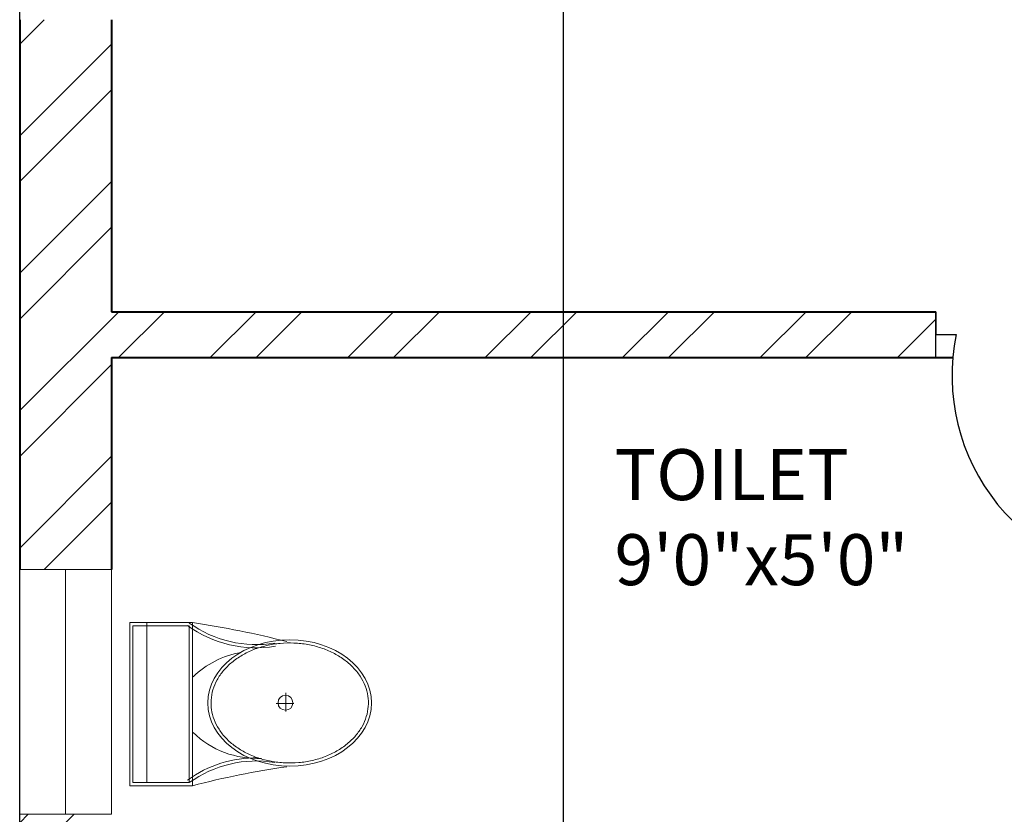
# Model space of a CAD drawing. Units: inches. Extents: x 1601 to 2297, y 1496 to 2631.
# Tile 6 of 57: x 1686 to 1783, y 1835 to 1913. Entities that reach past the tile are written whole.
import ezdxf

# ---------------------------------------------------------------- set-up
doc = ezdxf.new("R2010")
doc.units = ezdxf.units.IN
for name, color, linetype, lineweight in [('A-ANNO-DIMS', 2, 'Continuous', 18), ('A-AREA-IDEN', 7, 'Continuous', 18), ('A-DOOR', 21, 'Continuous', 25), ('A-FLOR-FIXT', 9, 'Continuous', 20), ('A-GLAZ', 161, 'Continuous', 20), ('A-WALL', 7, 'Continuous', 40), ('A-WALL-PATT', 215, 'Continuous', 13)]:
    doc.layers.add(name, color=color, linetype=linetype, lineweight=lineweight)
doc.styles.get("Standard").update_dxf_attribs({"font": 'arial.ttf'})
doc.dimstyles.get("Standard").update_dxf_attribs({"dimtxt": 0.18, "dimasz": 0.18, "dimexe": 0.18, "dimexo": 0.0625, "dimgap": 0.09, "dimtad": 0, "dimtih": 1, "dimtoh": 1, "dimdec": 4, "dimzin": 0, "dimdsep": 46, "dimtxsty": 'Standard', "dimcen": 0.09, "dimadec": 0, "dimazin": 0, "dimtfac": 1, "dimtdec": 4, "dimtofl": 0, "dimtmove": 0, "dimatfit": 3, "dimfxl": 1, "dimtolj": 1, "dimtzin": 0, "dimarcsym": 0})

# ---------------------------------------------------------------- blocks, each defined once
blk = doc.blocks.new('A$C31115884')
for p, q in [((257.5, 466.4), (257.5, 523.2)), ((283.1, 497.7), (223.4, 497.7)), ((0, 200), (0, 0)), ((520, 200), (0, 200)), ((10, 190), (10, 10)), ((510, 190), (10, 190)), ((510, 10), (510, 190)), ((520, 0), (520, 200)), ((510, 54.5), (0, 54.5)), ((10, 10), (510, 10)), ((0, 0), (520, 0))]:
    blk.add_line(p, q)
blk.add_circle((255.6, 496.4), 23.6)
for centre, radius, start, end in [((2777.7, -204.6), 2807, 165.4549, 171.7133), ((3237, 905), 2807, 188.2867, 194.5451), ((-294.5, 403.3), 364.7, 324.2091, 9.3499), ((-294.5, 403.3), 374.7, 324.2091, 9.3499), ((805.8, 403.3), 364.7, 170.6501, 215.7909), ((139.5, 406.2), 293.5, 315.8436, 2.6563), ((805.8, 403.3), 374.7, 179.2036, 215.7909), ((383.6, 406.2), 293.5, 190.2774, 224.1564)]:
    blk.add_arc(centre, radius, start, end)
blk.add_ellipse((256.2, 509.9), major_axis=(0, -260.7), ratio=0.772727)
blk.add_open_spline([(256.2, 259.2), (263.1, 259.2), (270, 259.7), (287.8, 262.3), (298.7, 265.1), (319.9, 273.1), (330.2, 278.4), (350.1, 291.1), (359.7, 298.7), (377.7, 315.9), (386.2, 325.5), (401.7, 346.6), (408.8, 358.1), (421.3, 382.5), (426.8, 395.5), (435.9, 422.4), (439.5, 436.4), (444.8, 465.1), (446.5, 479.7), (447.9, 509.2), (447.6, 524), (445, 553.3), (442.7, 567.8), (436.3, 596), (432.1, 609.7), (421.9, 636), (416, 648.6), (402.5, 672.1), (395, 683), (378.6, 703), (369.8, 712.1), (351.1, 728), (341.3, 734.8), (320.9, 746.2), (310.4, 750.7), (288.9, 757.3), (278, 759.4), (256, 761), (245, 760.6), (223.1, 757.2), (212.3, 754.3), (191.1, 746.1), (180.8, 740.7), (160.9, 727.8), (151.4, 720.1), (133.5, 702.7), (125.1, 693), (109.6, 671.7), (102.6, 660.2), (90.2, 635.7), (84.9, 622.7), (76, 595.6), (72.4, 581.6), (67.2, 552.9), (65.6, 538.2), (64.4, 508.8), (64.8, 494), (67.5, 464.7), (69.9, 450.2), (76.6, 422), (80.8, 408.3), (91.1, 382.2), (97.2, 369.7), (110.8, 346.3), (118.4, 335.4), (134.8, 315.6), (143.7, 306.7), (162.4, 290.9), (172.3, 284.2), (192.8, 273), (203.3, 268.6), (224.8, 262.2), (235.8, 260.2), (249.9, 259.3), (253, 259.2), (256.2, 259.2)], degree=3, knots=[0, 0, 0, 0, 0.110105, 0.110105, 0.285049, 0.285049, 0.459994, 0.459994, 0.634938, 0.634938, 0.809882, 0.809882, 0.984827, 0.984827, 1.159771, 1.159771, 1.334715, 1.334715, 1.50966, 1.50966, 1.684604, 1.684604, 1.859549, 1.859549, 2.034493, 2.034493, 2.209437, 2.209437, 2.384382, 2.384382, 2.559326, 2.559326, 2.73427, 2.73427, 2.909215, 2.909215, 3.084159, 3.084159, 3.259103, 3.259103, 3.434048, 3.434048, 3.608992, 3.608992, 3.783936, 3.783936, 3.958881, 3.958881, 4.133825, 4.133825, 4.30877, 4.30877, 4.483714, 4.483714, 4.658658, 4.658658, 4.833603, 4.833603, 5.008547, 5.008547, 5.183491, 5.183491, 5.358436, 5.358436, 5.53338, 5.53338, 5.708324, 5.708324, 5.883269, 5.883269, 6.058213, 6.058213, 6.233158, 6.233158, 6.283185, 6.283185, 6.283185, 6.283185])
blk = doc.blocks.new('WIN-24IN-JAMB9')
for p, q in [((4.5, 24), (0, 24)), ((0, 24), (9, 24)), ((0, 24), (0, 0)), ((4.5, 0), (4.5, 24)), ((9, 24), (9, 0)), ((0, 0), (9, 0)), ((9, 0), (4.5, 0))]:
    blk.add_line(p, q)
blk = doc.blocks.new('*D36')
at = {"layer": 'A-ANNO-DIMS', "color": 0, "lineweight": -2, "transparency": 16777216}
for p, q in [((1686.037, 1635.388), (1686.037, 2581.055)), ((1739.334, 1635.388), (1739.334, 2581.055)), ((1686.217, 2580.875), (1712.362, 2580.875)), ((1739.154, 2580.875), (1713.009, 2580.875))]:
    blk.add_line(p, q, dxfattribs=at)
at = {"layer": 'A-ANNO-DIMS', "color": 0, "transparency": 16777216}
for points in [[(1686.217, 2580.905), (1686.217, 2580.845), (1686.037, 2580.875)], [(1739.154, 2580.905), (1739.154, 2580.845), (1739.334, 2580.875)]]:
    blk.add_solid(points, dxfattribs=at)
at = {"layer": 'Defpoints', "color": 0, "transparency": 16777216}
for p in [(1739.334, 2580.875), (1686.037, 1635.325), (1739.334, 1635.325)]:
    blk.add_point(p, dxfattribs=at)
at = {"layer": 'A-ANNO-DIMS', "color": 0, "transparency": 16777216, "insert": (1712.685, 2580.875), "char_height": 0.18, "attachment_point": 5}
blk.add_mtext('\\A1;53.3', dxfattribs=at)

msp = doc.modelspace()

# ---------------------------------------------------------------- hatches: boundary and pattern name
at = {"layer": 'A-WALL-PATT'}
h = msp.add_hatch(dxfattribs=at)
h.set_pattern_fill('ANSI32', color=256)
h.paths.add_polyline_path([(1842.0336, 2528.0767), (1842.0336, 2532.3254), (1686.0373, 2532.3254), (1686.0373, 2492.9493), (1695.0373, 2492.9493), (1695.0373, 2523.3254), (1827.0373, 2523.3254), (1827.0373, 2416.8254), (1834.6225, 2416.8254), (1834.6225, 2419.0754), (1834.6225, 2421.3254), (1831.5373, 2421.3254), (1831.5373, 2523.3254), (1842.0336, 2523.3254)])
h.paths.add_polyline_path([(1695.0373, 2432.9493), (1686.0373, 2432.9493), (1686.0373, 2325.989), (1695.0373, 2325.989), (1695.0373, 2347.8254), (1827.0373, 2347.8254), (1827.0373, 2287.8254), (1823.2991, 2287.8254), (1823.2991, 2283.3254), (1847.9422, 2283.3254), (1847.9422, 2285.5754), (1847.9422, 2287.8254), (1831.5373, 2287.8254), (1831.5373, 2347.8254), (1846.9946, 2347.8254), (1846.9946, 2350.0754), (1846.9946, 2352.3254), (1695.0373, 2352.3254)])
h.paths.add_polyline_path([(1807.1169, 1573.5395), (2055.0405, 1573.5395), (2055.0405, 1610.6322), (1807.1169, 1610.6322)], flags=9)
h.paths.add_polyline_path([(1841.1631, 1712.7967), (1870.3957, 1712.7967), (1870.3957, 1731.454), (1841.1631, 1731.454)], flags=9)
h.paths.add_polyline_path([(2144.3862, 1772.185), (2191.0233, 1772.185), (2191.0233, 1790.8423), (2144.3862, 1790.8423)], flags=9)
h.paths.add_polyline_path([(2143.0128, 1827.3312), (2177.9958, 1827.3312), (2177.9958, 1845.9886), (2143.0128, 1845.9886)], flags=9)
h.paths.add_polyline_path([(2041.2439, 1833.5691), (2070.8516, 1833.5691), (2070.8516, 1852.2264), (2041.2439, 1852.2264)], flags=9)
h.paths.add_polyline_path([(2097.2791, 1947.0598), (2134.2061, 1947.0598), (2134.2061, 1965.7171), (2097.2791, 1965.7171)], flags=9)
h.paths.add_polyline_path([(2214.995, 1904.3124), (2214.995, 1942.2899), (2196.3376, 1942.2899), (2196.3376, 1904.3124)], flags=9)
h.paths.add_polyline_path([(2186.6284, 2043.8031), (2219.7935, 2043.8031), (2219.7935, 2062.4605), (2186.6284, 2062.4605)], flags=9)
h.paths.add_polyline_path([(2064.0877, 2031.616), (2097.4949, 2031.616), (2097.4949, 2050.2734), (2064.0877, 2050.2734)], flags=9)
h.paths.add_polyline_path([(1973.1349, 1986.0688), (2008.4009, 1986.0688), (2008.4009, 2004.7261), (1973.1349, 2004.7261)], flags=9)
h.paths.add_polyline_path([(1976.3676, 2106.9635), (2005.7469, 2106.9635), (2005.7469, 2125.6209), (1976.3676, 2125.6209)], flags=9)
h.paths.add_polyline_path([(1991.7852, 2180.4863), (2027.0513, 2180.4863), (2027.0513, 2199.1437), (1991.7852, 2199.1437)], flags=9)
h.paths.add_polyline_path([(2106.1801, 2187.9359), (2152.2101, 2187.9359), (2152.2101, 2206.5932), (2106.1801, 2206.5932)], flags=9)
h.paths.add_polyline_path([(2148.6686, 2262.2542), (2182.318, 2262.2542), (2182.318, 2280.9115), (2148.6686, 2280.9115)], flags=9)
h.paths.add_polyline_path([(2041.6327, 2252.8147), (2071.2405, 2252.8147), (2071.2405, 2271.4721), (2041.6327, 2271.4721)], flags=9)
h.paths.add_polyline_path([(2063.9734, 2375.4265), (2100.9004, 2375.4265), (2100.9004, 2394.0839), (2063.9734, 2394.0839)], flags=9)
h.paths.add_polyline_path([(2216.4955, 2330.9748), (2216.4955, 2370.2654), (2197.8381, 2370.2654), (2197.8381, 2330.9748)], flags=9)
h.paths.add_polyline_path([(2179.1416, 2485.8687), (2212.3067, 2485.8687), (2212.3067, 2504.5261), (2179.1416, 2504.5261)], flags=9)
h.paths.add_polyline_path([(2078.7442, 2471.1516), (2112.1514, 2471.1516), (2112.1514, 2489.809), (2078.7442, 2489.809)], flags=9)
h.paths.add_polyline_path([(1915.9631, 2329.4668), (1952.8902, 2329.4668), (1952.8902, 2348.1241), (1915.9631, 2348.1241)], flags=9)
h.paths.add_polyline_path([(1904.3189, 2499.6709), (1940.4512, 2499.6709), (1940.4512, 2518.3282), (1904.3189, 2518.3282)], flags=9)
h.paths.add_polyline_path([(1892.3665, 2100.4595), (1925.6374, 2100.4595), (1925.6374, 2119.1169), (1892.3665, 2119.1169)], flags=9)
h.paths.add_polyline_path([(1909.2984, 1805.9631), (1946.2254, 1805.9631), (1946.2254, 1824.6205), (1909.2984, 1824.6205)], flags=9)
h.paths.add_polyline_path([(1934.6056, 1658.616), (1970.738, 1658.616), (1970.738, 1677.2733), (1934.6056, 1677.2733)], flags=9)
h.paths.add_polyline_path([(1711.2052, 1789.8902), (1750.0456, 1789.8902), (1750.0456, 1808.5476), (1711.2052, 1808.5476)], flags=9)
h.paths.add_polyline_path([(1742.7874, 1854.6743), (1771.9449, 1854.6743), (1771.9449, 1873.3317), (1742.7874, 1873.3317)], flags=9)
h.paths.add_polyline_path([(1807.3592, 1997.7912), (1850.1116, 1997.7912), (1850.1116, 2016.4486), (1807.3592, 2016.4486)], flags=9)
h.paths.add_polyline_path([(1717.4579, 2237.7844), (1760.2103, 2237.7844), (1760.2103, 2256.4417), (1717.4579, 2256.4417)], flags=9)
h.paths.add_polyline_path([(1780.9285, 2324.0623), (1810.086, 2324.0623), (1810.086, 2342.7197), (1780.9285, 2342.7197)], flags=25)
h.paths.add_polyline_path([(1837.696, 2449.2024), (1866.9286, 2449.2024), (1866.9286, 2467.8598), (1837.696, 2467.8598)], flags=9)
h.paths.add_polyline_path([(1712.7752, 2484.9404), (1751.6156, 2484.9404), (1751.6156, 2503.5977), (1712.7752, 2503.5977)], flags=25)
h = msp.add_hatch(dxfattribs=at)
h.set_pattern_fill('ANSI32', color=256)
h.paths.add_polyline_path([(1973.9371, 2211.3254), (1893.0373, 2211.3254), (1893.0373, 2287.8254), (1884.6167, 2287.8254), (1884.6167, 2285.5754), (1884.6167, 2283.3254), (1888.5373, 2283.3254), (1888.5373, 2145.3254), (1695.0373, 2145.3254), (1695.0373, 2173.8724), (1690.5373, 2173.8724), (1686.0373, 2173.8724), (1686.0373, 2136.3254), (1722.5687, 2136.3254), (1722.5687, 2117.4352), (1731.5687, 2117.4352), (1731.5687, 2136.3254), (1893.0373, 2136.3254), (1893.0373, 2202.3254), (1959.0373, 2202.3254), (1959.0373, 2182.1303), (1968.0373, 2182.1303), (1968.0373, 2202.3254), (1973.9371, 2202.3254)])
h.paths.add_polyline_path([(2094.0373, 2274.6364), (2096.4294, 2274.6364), (2096.4294, 2276.8864), (2096.4294, 2279.1364), (2094.0373, 2279.1364), (2094.0373, 2290.8254), (2094.0373, 2295.3254), (2089.5373, 2295.3254), (2089.5373, 2230.8254), (2035.5373, 2230.8254), (2035.5373, 2299.8254), (2031.0373, 2299.8254), (2031.0373, 2211.3254), (2023.0065, 2211.3254), (2023.0065, 2202.3254), (2031.0373, 2202.3254), (2031.0373, 2140.8254), (1968.0373, 2140.8254), (1968.0373, 2145.9106), (1963.5373, 2145.9106), (1959.0373, 2145.9106), (1959.0373, 2116.839), (1963.5373, 2116.839), (1968.0373, 2116.839), (1968.0373, 2131.8254), (2031.0373, 2131.8254), (2031.0373, 2094.3254), (2031.0373, 2085.3254), (2031.0373, 2056.8254), (1968.0373, 2056.8254), (1968.0373, 2070.4947), (1963.5373, 2070.4947), (1959.0373, 2070.4947), (1959.0373, 2040.3029), (1968.0373, 2040.3029), (1968.0373, 2047.8254), (2031.0373, 2047.8254), (2031.0373, 1983.3254), (2031.0373, 1978.8254), (2021.1979, 1978.8254), (2021.1979, 1974.3254), (2031.0373, 1974.3254), (2031.0373, 1954.3528), (2035.5373, 1954.3528), (2035.5373, 1974.3254), (2035.5373, 1981.8254), (2055.5513, 1981.8254), (2055.5513, 1986.3254), (2035.5373, 1986.3254), (2035.5373, 2047.8254), (2040.0373, 2047.8254), (2040.0373, 2085.3254), (2040.0373, 2094.3254), (2040.0373, 2140.8254), (2035.5373, 2140.8254), (2035.5373, 2226.3254), (2089.5373, 2226.3254), (2094.0373, 2226.3254)])
h.paths.add_polyline_path([(2226.0373, 2230.8254), (2134.5373, 2230.8254), (2134.5373, 2233.5437), (2130.0373, 2233.5437), (2130.0373, 2226.3254), (2134.5373, 2226.3254), (2226.0373, 2226.3254)])
h.paths.add_polyline_path([(1807.1169, 1573.5395), (2055.0405, 1573.5395), (2055.0405, 1610.6322), (1807.1169, 1610.6322)], flags=9)
h.paths.add_polyline_path([(1841.1631, 1712.7967), (1870.3957, 1712.7967), (1870.3957, 1731.454), (1841.1631, 1731.454)], flags=9)
h.paths.add_polyline_path([(2144.3862, 1772.185), (2191.0233, 1772.185), (2191.0233, 1790.8423), (2144.3862, 1790.8423)], flags=9)
h.paths.add_polyline_path([(2143.0128, 1827.3312), (2177.9958, 1827.3312), (2177.9958, 1845.9886), (2143.0128, 1845.9886)], flags=9)
h.paths.add_polyline_path([(2041.2439, 1833.5691), (2070.8516, 1833.5691), (2070.8516, 1852.2264), (2041.2439, 1852.2264)], flags=9)
h.paths.add_polyline_path([(2097.2791, 1947.0598), (2134.2061, 1947.0598), (2134.2061, 1965.7171), (2097.2791, 1965.7171)], flags=9)
h.paths.add_polyline_path([(2214.995, 1904.3124), (2214.995, 1942.2899), (2196.3376, 1942.2899), (2196.3376, 1904.3124)], flags=9)
h.paths.add_polyline_path([(2186.6284, 2043.8031), (2219.7935, 2043.8031), (2219.7935, 2062.4605), (2186.6284, 2062.4605)], flags=9)
h.paths.add_polyline_path([(2064.0877, 2031.616), (2097.4949, 2031.616), (2097.4949, 2050.2734), (2064.0877, 2050.2734)], flags=9)
h.paths.add_polyline_path([(1973.1349, 1986.0688), (2008.4009, 1986.0688), (2008.4009, 2004.7261), (1973.1349, 2004.7261)], flags=25)
h.paths.add_polyline_path([(1976.3676, 2106.9635), (2005.7469, 2106.9635), (2005.7469, 2125.6209), (1976.3676, 2125.6209)], flags=25)
h.paths.add_polyline_path([(1991.7852, 2180.4863), (2027.0513, 2180.4863), (2027.0513, 2199.1437), (1991.7852, 2199.1437)], flags=25)
h.paths.add_polyline_path([(2106.1801, 2187.9359), (2152.2101, 2187.9359), (2152.2101, 2206.5932), (2106.1801, 2206.5932)], flags=9)
h.paths.add_polyline_path([(2148.6686, 2262.2542), (2182.318, 2262.2542), (2182.318, 2280.9115), (2148.6686, 2280.9115)], flags=9)
h.paths.add_polyline_path([(2041.6327, 2252.8147), (2071.2405, 2252.8147), (2071.2405, 2271.4721), (2041.6327, 2271.4721)], flags=25)
h.paths.add_polyline_path([(2063.9734, 2375.4265), (2100.9004, 2375.4265), (2100.9004, 2394.0839), (2063.9734, 2394.0839)], flags=9)
h.paths.add_polyline_path([(2216.4955, 2330.9748), (2216.4955, 2370.2654), (2197.8381, 2370.2654), (2197.8381, 2330.9748)], flags=9)
h.paths.add_polyline_path([(2179.1416, 2485.8687), (2212.3067, 2485.8687), (2212.3067, 2504.5261), (2179.1416, 2504.5261)], flags=9)
h.paths.add_polyline_path([(2078.7442, 2471.1516), (2112.1514, 2471.1516), (2112.1514, 2489.809), (2078.7442, 2489.809)], flags=9)
h.paths.add_polyline_path([(1915.9631, 2329.4668), (1952.8902, 2329.4668), (1952.8902, 2348.1241), (1915.9631, 2348.1241)], flags=9)
h.paths.add_polyline_path([(1904.3189, 2499.6709), (1940.4512, 2499.6709), (1940.4512, 2518.3282), (1904.3189, 2518.3282)], flags=9)
h.paths.add_polyline_path([(1892.3665, 2100.4595), (1925.6374, 2100.4595), (1925.6374, 2119.1169), (1892.3665, 2119.1169)], flags=9)
h.paths.add_polyline_path([(1909.2984, 1805.9631), (1946.2254, 1805.9631), (1946.2254, 1824.6205), (1909.2984, 1824.6205)], flags=9)
h.paths.add_polyline_path([(1934.6056, 1658.616), (1970.738, 1658.616), (1970.738, 1677.2733), (1934.6056, 1677.2733)], flags=9)
h.paths.add_polyline_path([(1711.2052, 1789.8902), (1750.0456, 1789.8902), (1750.0456, 1808.5476), (1711.2052, 1808.5476)], flags=9)
h.paths.add_polyline_path([(1742.7874, 1854.6743), (1771.9449, 1854.6743), (1771.9449, 1873.3317), (1742.7874, 1873.3317)], flags=9)
h.paths.add_polyline_path([(1807.3592, 1997.7912), (1850.1116, 1997.7912), (1850.1116, 2016.4486), (1807.3592, 2016.4486)], flags=9)
h.paths.add_polyline_path([(1717.4579, 2237.7844), (1760.2103, 2237.7844), (1760.2103, 2256.4417), (1717.4579, 2256.4417)], flags=25)
h.paths.add_polyline_path([(1780.9285, 2324.0623), (1810.086, 2324.0623), (1810.086, 2342.7197), (1780.9285, 2342.7197)], flags=9)
h.paths.add_polyline_path([(1837.696, 2449.2024), (1866.9286, 2449.2024), (1866.9286, 2467.8598), (1837.696, 2467.8598)], flags=9)
h.paths.add_polyline_path([(1712.7752, 2484.9404), (1751.6156, 2484.9404), (1751.6156, 2503.5977), (1712.7752, 2503.5977)], flags=9)
h = msp.add_hatch(dxfattribs=at)
h.set_pattern_fill('ANSI32', color=256)
h.paths.add_polyline_path([(2230.5373, 1861.8254), (2182.5373, 1861.8254), (2182.5373, 1885.3637), (2178.0373, 1885.3637), (2178.0373, 1861.8254), (2166.0373, 1861.8254), (2134.5373, 1861.8254), (2130.0373, 1861.8254), (2130.0373, 1841.4682), (2126.8833, 1841.4682), (2126.8833, 1836.9682), (2130.0373, 1836.9682), (2130.0373, 1822.7302), (2134.5373, 1822.7302), (2134.5373, 1857.3254), (2166.0373, 1857.3254), (2226.0373, 1857.3254), (2226.0373, 1846.1155), (2230.5373, 1846.1155)])
h.paths.add_polyline_path([(2226.0373, 1797.3254), (2134.5373, 1797.3254), (2134.5373, 1800.6636), (2132.2873, 1800.6636), (2130.0373, 1800.6636), (2130.0373, 1797.3254), (2130.0373, 1792.8254), (2167.7264, 1792.8254), (2226.0373, 1792.8254)])
h.paths.add_polyline_path([(2230.5373, 1822.1155), (2226.0373, 1822.1155), (2226.0373, 1760.8563), (2230.5373, 1760.8563)])
h.paths.add_polyline_path([(2230.5373, 1700.8563), (2226.0373, 1700.8563), (2226.0373, 1644.3254), (2140.2517, 1644.3254), (2140.2517, 1635.3254), (2230.5373, 1635.3254)])
h.paths.add_polyline_path([(2080.2517, 1639.8254), (2080.2517, 1644.3254), (2035.5373, 1644.3254), (2035.5373, 1792.8254), (2094.0373, 1792.8254), (2094.0373, 1797.3254), (2094.0373, 1836.9682), (2097.1057, 1836.9682), (2097.1057, 1839.2182), (2097.1057, 1841.4682), (2094.0373, 1841.4682), (2094.0373, 1862.2276), (2089.5373, 1862.2276), (2089.5373, 1797.3254), (2035.5373, 1797.3254), (2035.5373, 1857.3254), (2035.5373, 1885.0916), (2031.0373, 1885.0916), (2031.0373, 1710.3254), (2012.329, 1710.3254), (2012.329, 1701.3254), (2031.0373, 1701.3254), (2031.0373, 1644.3254), (2031.0373, 1635.3254), (2080.2517, 1635.3254)])
h.paths.add_polyline_path([(1836.0373, 1653.2033), (1842.6171, 1653.2033), (1842.6171, 1657.7033), (1842.6171, 1662.2033), (1831.5373, 1662.2033), (1831.5373, 1764.2033), (1835.3881, 1764.2033), (1835.3881, 1766.4533), (1835.3881, 1768.7033), (1831.5373, 1768.7033), (1827.0373, 1768.7033), (1827.0373, 1662.2033), (1827.0373, 1635.3254), (1836.0373, 1635.3254)])
h.paths.add_polyline_path([(1893.0373, 1701.3254), (1907.193, 1701.3254), (1907.193, 1705.8254), (1907.193, 1710.3254), (1893.0373, 1710.3254), (1893.0373, 1819.8254), (1882.6444, 1819.8254), (1882.6444, 1817.5754), (1882.6444, 1815.3254), (1888.5373, 1815.3254), (1888.5373, 1662.2033), (1884.0373, 1662.2033), (1866.6171, 1662.2033), (1866.6171, 1653.2033), (1882.391, 1653.2033), (1884.0373, 1653.2033), (1884.0373, 1635.3254), (1893.0373, 1635.3254)])
h.paths.add_polyline_path([(1739.3335, 1639.8254), (1739.3335, 1644.3254), (1695.0373, 1644.3254), (1695.0373, 1702.0135), (1690.5373, 1702.0135), (1686.0373, 1702.0135), (1686.0373, 1635.3254), (1739.3335, 1635.3254)])
h.paths.add_polyline_path([(1827.0373, 1644.3254), (1799.3335, 1644.3254), (1799.3335, 1635.3254), (1827.0373, 1635.3254)])
h.paths.add_polyline_path([(1695.0373, 1815.3254), (1849.2759, 1815.3254), (1849.2759, 1819.8254), (1807.5373, 1819.8254), (1807.5373, 1879.8254), (1851.1533, 1879.8254), (1851.1533, 1882.0754), (1851.1533, 1884.3254), (1799.3405, 1884.3254), (1799.3405, 1882.0754), (1799.3405, 1879.8254), (1803.0373, 1879.8254), (1803.0373, 1819.8254), (1695.0373, 1819.8254), (1695.0373, 1835.0458), (1690.5373, 1835.0458), (1686.0373, 1835.0458), (1686.0373, 1766.1753), (1695.0373, 1766.1753)])
h.paths.add_polyline_path([(1775.8157, 1884.3254), (1695.0373, 1884.3254), (1695.0373, 1912.9526), (1690.5373, 1912.9526), (1686.0373, 1912.9526), (1686.0373, 1859.0458), (1695.0373, 1859.0458), (1695.0373, 1879.8254), (1775.8157, 1879.8254)])
h.paths.add_polyline_path([(1893.0373, 2031.3254), (1731.5687, 2031.3254), (1731.5687, 2057.4352), (1722.5687, 2057.4352), (1722.5687, 2031.3254), (1686.0373, 2031.3254), (1686.0373, 1972.9526), (1695.0373, 1972.9526), (1695.0373, 2022.3254), (1888.5373, 2022.3254), (1888.5373, 1884.3254), (1883.4996, 1884.3254), (1883.4996, 1879.8254), (1893.0373, 1879.8254), (1893.0373, 1974.3254), (1976.6199, 1974.3254), (1976.6199, 1978.8254), (1968.0373, 1978.8254), (1968.0373, 1983.3254), (1968.0373, 2008.4756), (1963.5373, 2008.4756), (1959.0373, 2008.4756), (1959.0373, 1983.3254), (1893.0373, 1983.3254)])
h.paths.add_polyline_path([(2230.5373, 2140.4745), (2226.0373, 2140.4745), (2226.0373, 2094.3254), (2040.0373, 2094.3254), (2040.0373, 2085.3254), (2178.0373, 2085.3254), (2178.0373, 2065.6965), (2182.5373, 2065.6965), (2182.5373, 2085.3254), (2226.0373, 2085.3254), (2226.0373, 1986.3254), (2211.2679, 1986.3254), (2211.2679, 1981.8254), (2230.5373, 1981.8254)])
h.paths.add_polyline_path([(2187.6292, 1986.3254), (2182.5373, 1986.3254), (2182.5373, 2029.6965), (2178.0373, 2029.6965), (2178.0373, 1986.3254), (2099.05, 1986.3254), (2099.05, 1981.8254), (2178.0373, 1981.8254), (2178.0373, 1969.3637), (2182.5373, 1969.3637), (2182.5373, 1981.8254), (2187.6292, 1981.8254), (2187.6292, 1984.0754)])
h.paths.add_polyline_path([(1807.1169, 1573.5395), (2055.0405, 1573.5395), (2055.0405, 1610.6322), (1807.1169, 1610.6322)], flags=9)
h.paths.add_polyline_path([(1841.1631, 1712.7967), (1870.3957, 1712.7967), (1870.3957, 1731.454), (1841.1631, 1731.454)], flags=9)
h.paths.add_polyline_path([(2144.3862, 1772.185), (2191.0233, 1772.185), (2191.0233, 1790.8423), (2144.3862, 1790.8423)], flags=9)
h.paths.add_polyline_path([(2143.0128, 1827.3312), (2177.9958, 1827.3312), (2177.9958, 1845.9886), (2143.0128, 1845.9886)], flags=25)
h.paths.add_polyline_path([(2041.2439, 1833.5691), (2070.8516, 1833.5691), (2070.8516, 1852.2264), (2041.2439, 1852.2264)], flags=25)
h.paths.add_polyline_path([(2097.2791, 1947.0598), (2134.2061, 1947.0598), (2134.2061, 1965.7171), (2097.2791, 1965.7171)], flags=9)
h.paths.add_polyline_path([(2214.995, 1904.3124), (2214.995, 1942.2899), (2196.3376, 1942.2899), (2196.3376, 1904.3124)], flags=9)
h.paths.add_polyline_path([(2186.6284, 2043.8031), (2219.7935, 2043.8031), (2219.7935, 2062.4605), (2186.6284, 2062.4605)], flags=25)
h.paths.add_polyline_path([(2064.0877, 2031.616), (2097.4949, 2031.616), (2097.4949, 2050.2734), (2064.0877, 2050.2734)], flags=25)
h.paths.add_polyline_path([(1973.1349, 1986.0688), (2008.4009, 1986.0688), (2008.4009, 2004.7261), (1973.1349, 2004.7261)], flags=9)
h.paths.add_polyline_path([(1976.3676, 2106.9635), (2005.7469, 2106.9635), (2005.7469, 2125.6209), (1976.3676, 2125.6209)], flags=9)
h.paths.add_polyline_path([(1991.7852, 2180.4863), (2027.0513, 2180.4863), (2027.0513, 2199.1437), (1991.7852, 2199.1437)], flags=9)
h.paths.add_polyline_path([(2106.1801, 2187.9359), (2152.2101, 2187.9359), (2152.2101, 2206.5932), (2106.1801, 2206.5932)], flags=9)
h.paths.add_polyline_path([(2148.6686, 2262.2542), (2182.318, 2262.2542), (2182.318, 2280.9115), (2148.6686, 2280.9115)], flags=9)
h.paths.add_polyline_path([(2041.6327, 2252.8147), (2071.2405, 2252.8147), (2071.2405, 2271.4721), (2041.6327, 2271.4721)], flags=9)
h.paths.add_polyline_path([(2063.9734, 2375.4265), (2100.9004, 2375.4265), (2100.9004, 2394.0839), (2063.9734, 2394.0839)], flags=9)
h.paths.add_polyline_path([(2216.4955, 2330.9748), (2216.4955, 2370.2654), (2197.8381, 2370.2654), (2197.8381, 2330.9748)], flags=9)
h.paths.add_polyline_path([(2179.1416, 2485.8687), (2212.3067, 2485.8687), (2212.3067, 2504.5261), (2179.1416, 2504.5261)], flags=9)
h.paths.add_polyline_path([(2078.7442, 2471.1516), (2112.1514, 2471.1516), (2112.1514, 2489.809), (2078.7442, 2489.809)], flags=9)
h.paths.add_polyline_path([(1915.9631, 2329.4668), (1952.8902, 2329.4668), (1952.8902, 2348.1241), (1915.9631, 2348.1241)], flags=9)
h.paths.add_polyline_path([(1904.3189, 2499.6709), (1940.4512, 2499.6709), (1940.4512, 2518.3282), (1904.3189, 2518.3282)], flags=9)
h.paths.add_polyline_path([(1892.3665, 2100.4595), (1925.6374, 2100.4595), (1925.6374, 2119.1169), (1892.3665, 2119.1169)], flags=9)
h.paths.add_polyline_path([(1909.2984, 1805.9631), (1946.2254, 1805.9631), (1946.2254, 1824.6205), (1909.2984, 1824.6205)], flags=9)
h.paths.add_polyline_path([(1934.6056, 1658.616), (1970.738, 1658.616), (1970.738, 1677.2733), (1934.6056, 1677.2733)], flags=9)
h.paths.add_polyline_path([(1711.2052, 1789.8902), (1750.0456, 1789.8902), (1750.0456, 1808.5476), (1711.2052, 1808.5476)], flags=25)
h.paths.add_polyline_path([(1742.7874, 1854.6743), (1771.9449, 1854.6743), (1771.9449, 1873.3317), (1742.7874, 1873.3317)], flags=25)
h.paths.add_polyline_path([(1807.3592, 1997.7912), (1850.1116, 1997.7912), (1850.1116, 2016.4486), (1807.3592, 2016.4486)], flags=25)
h.paths.add_polyline_path([(1717.4579, 2237.7844), (1760.2103, 2237.7844), (1760.2103, 2256.4417), (1717.4579, 2256.4417)], flags=9)
h.paths.add_polyline_path([(1780.9285, 2324.0623), (1810.086, 2324.0623), (1810.086, 2342.7197), (1780.9285, 2342.7197)], flags=9)
h.paths.add_polyline_path([(1837.696, 2449.2024), (1866.9286, 2449.2024), (1866.9286, 2467.8598), (1837.696, 2467.8598)], flags=9)
h.paths.add_polyline_path([(1712.7752, 2484.9404), (1751.6156, 2484.9404), (1751.6156, 2503.5977), (1712.7752, 2503.5977)], flags=9)

# ---------------------------------------------------------------- linework, layer by layer
at = {"layer": 'A-DOOR'}
for p, q in [((1775.8157, 1879.8254), (1775.8157, 1884.3254)), ((1775.8157, 1884.3254), (1775.8157, 1882.0754)), ((1775.8157, 1882.0754), (1777.8157, 1882.0754))]:
    msp.add_line(p, q, dxfattribs=at)
msp.add_arc((1797.3405, 1878.0174), 19.942, 168.258947, 270, dxfattribs=at)
at = {"layer": 'A-WALL'}
for p, q in [((1686.0373, 1912.9526), (1686.0373, 1859.0458)), ((1695.0373, 1912.9526), (1695.0373, 1884.3254)), ((1695.0373, 1884.3254), (1775.8157, 1884.3254)), ((1695.0373, 1879.8254), (1777.4806, 1879.8254)), ((1695.0373, 1879.8254), (1777.4806, 1879.8254)), ((1695.0373, 1879.8254), (1695.0373, 1859.0458))]:
    msp.add_line(p, q, dxfattribs=at)

# ---------------------------------------------------------------- block references
at = {"layer": 'A-FLOR-FIXT', "xscale": 0.0307498789965588, "yscale": 0.0307498789965588, "zscale": 0.0307498789965588, "rotation": 270}
msp.add_blockref('A$C31115884', (1696.8178, 1853.8393), dxfattribs=at)
at = {"layer": 'A-GLAZ'}
msp.add_blockref('WIN-24IN-JAMB9', (1686.037, 1835.046), dxfattribs=at)

# ---------------------------------------------------------------- texts
at = {"layer": 'A-AREA-IDEN', "insert": (1744.3273, 1870.847), "char_height": 5, "attachment_point": 1}
msp.add_mtext_dynamic_manual_height_columns('TOILET\\P9\'0"x5\'0"', width=79.077705, gutter_width=12.5, heights=[0], dxfattribs=at)

# ---------------------------------------------------------------- dimensions: what is measured, and where the dimension line sits
at = {"layer": 'A-ANNO-DIMS'}
dim = msp.add_linear_dim(base=(1739.3335, 2580.8754), p1=(1686.0373, 1635.3254), p2=(1739.3335, 1635.3254), dimstyle='Standard', override={"dimdec": 1, "dimlfac": 1, "dimrnd": 0, "dimzin": 0, "dimdsep": 46, "dimlunit": 2}, dxfattribs=at)
dim.commit()
dim.dimension.update_dxf_attribs({"geometry": '*D36', "text_midpoint": (1712.6854, 2580.8754)})

doc.saveas('drawing.dxf')
